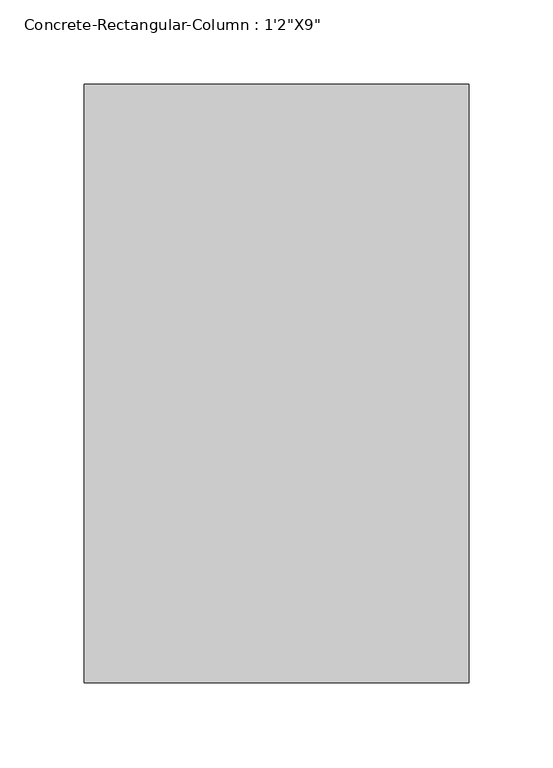
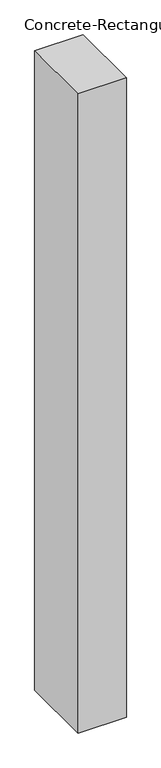
"""IFC4 building model written with IfcOpenShell, lengths in millimetres: column geometry."""

from ifc_helpers import new_model, si_unit, origin, origin_with_axes, place, context, project, spatial, polyline, outline, extrude, source, transform, mapped, element, save


def column_add0f710(model_context):
    return source(origin(), model_context, "Body", "SweptSolid", [
        extrude(outline(polyline([(114.3, 177.8), (114.3, -177.8), (-114.3, -177.8), (-114.3, 177.8), (114.3, 177.8)])), origin_with_axes(), (0.0, 0.0, 1.0), 3200.4),
    ])


if __name__ == "__main__":
    model = new_model("IFC4")
    model_context = context("Model", 3, world=origin())
    ifc_project = project(units=[si_unit("LENGTHUNIT", "METRE", prefix="MILLI")], contexts=[model_context])
    site = spatial("IfcSite", under=ifc_project)
    building = spatial("IfcBuilding", under=site)
    placement = place(None, origin())
    column_shape = column_add0f710(model_context)
    element("IfcColumn", 1, ObjectType="Concrete-Rectangular-Column : 1'2\"X9\"", at=placement, inside=building, context=model_context, shape_type="MappedRepresentation", body=[
        mapped(column_shape, transform((0.0, 0.0, 0.0), x_axis=(1.0, 0.0, 0.0), y_axis=(0.0, 1.0, 0.0), z_axis=(0.0, 0.0, 1.0))),
    ])
    save(model, "model.ifc")

# Revit data of these elements
# Type "Concrete-Rectangular-Column : 1'2\"X9\""
#   Assembly Code = "B10"
#   b = 0' - 9"
#   h = 1' - 2"
#   Structural Material [instance default] = Concrete, Cast-in-Place gray
# Element 1 (IfcColumn, "Concrete-Rectangular-Column : 1'2\"X9\"")
#   Materials on its faces: "Concrete, Cast-in-Place gray"
# Materials
#   "Concrete, Cast-in-Place gray": class "Concrete", colour RGB 192 192 192, transparency 0, Description = "Cast-in-place concrete", Cost = 0
